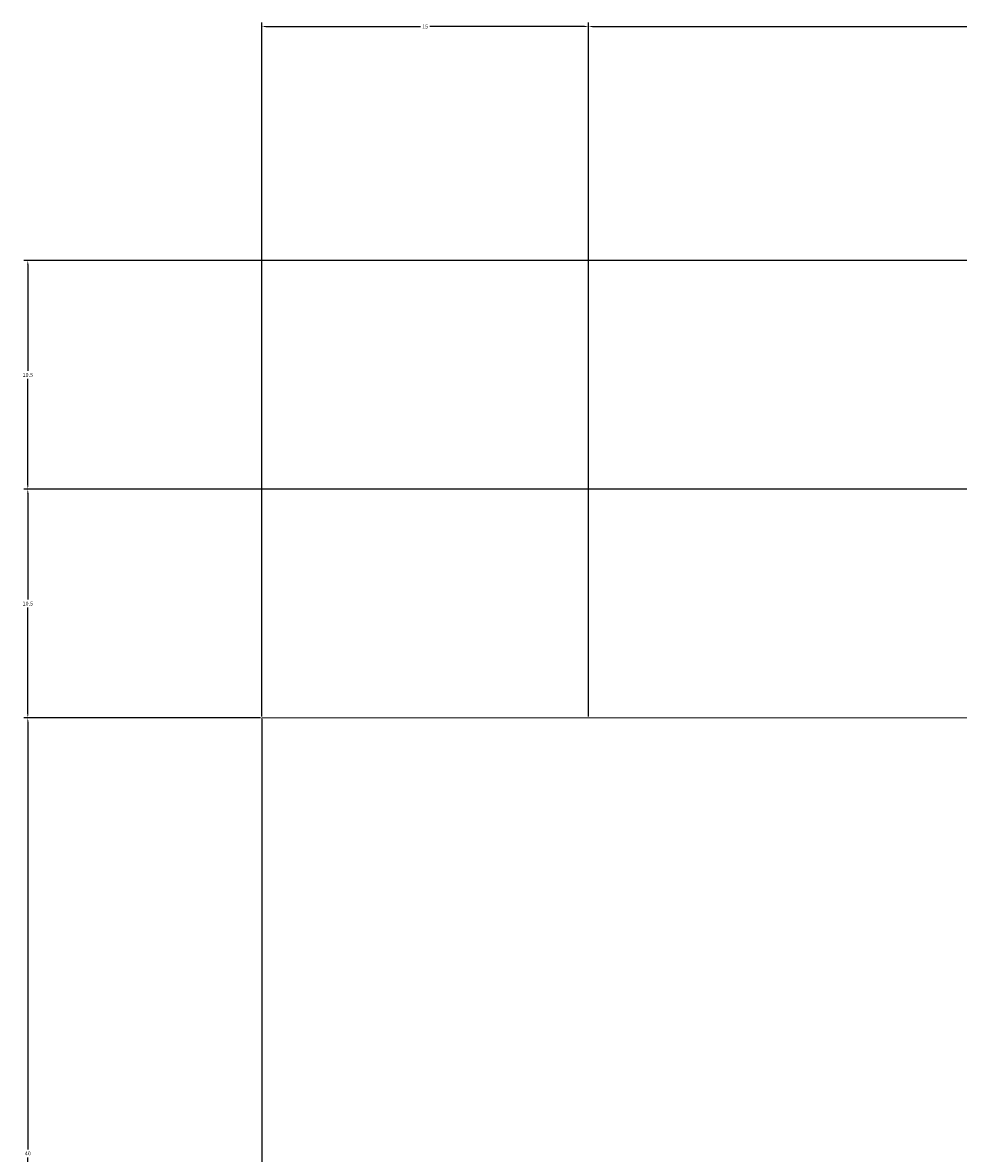
# Model space of a CAD drawing. Units: millimetres. Extents: x 315 to 487, y -72 to 32.
# Tile 2 of 4: x 315 to 358, y -20 to 32. Entities that reach past the tile are written whole.
import ezdxf

# ---------------------------------------------------------------- set-up
doc = ezdxf.new("R2010")
doc.units = ezdxf.units.MM
doc.layers.add('M-CONS', color=8, linetype='Continuous', lineweight=13)
doc.layers.add('M-DIMS', color=2, linetype='Continuous', lineweight=18)
doc.styles.get("Standard").update_dxf_attribs({"font": 'arial.ttf'})
doc.dimstyles.get("Standard").update_dxf_attribs({"dimtxt": 0.18, "dimasz": 0.18, "dimexe": 0.18, "dimexo": 0.0625, "dimgap": 0.09, "dimtad": 0, "dimtih": 1, "dimtoh": 1, "dimdec": 4, "dimzin": 0, "dimdsep": 46, "dimtxsty": 'Standard', "dimcen": 0.09, "dimadec": 0, "dimazin": 0, "dimtfac": 1, "dimtdec": 4, "dimtofl": 0, "dimtmove": 0, "dimatfit": 3, "dimfxl": 1, "dimtolj": 1, "dimtzin": 0, "dimarcsym": 0})

# ---------------------------------------------------------------- blocks, each defined once
blk = doc.blocks.new('*D3')
at = {"layer": 'Defpoints', "color": 0, "transparency": 16777216}
for p in [(326.007, 0), (476.007, 0), (476.007, -71.75)]:
    blk.add_point(p, dxfattribs=at)
at = {"layer": 'M-DIMS', "color": 0, "lineweight": -2, "transparency": 16777216}
for p, q in [((326.007, -0.062), (326.007, -71.93)), ((476.007, -0.062), (476.007, -71.93)), ((326.187, -71.75), (400.727, -71.75)), ((475.827, -71.75), (401.287, -71.75))]:
    blk.add_line(p, q, dxfattribs=at)
at = {"layer": 'M-DIMS', "color": 0, "transparency": 16777216}
for points in [[(326.187, -71.72), (326.187, -71.78), (326.007, -71.75)], [(475.827, -71.72), (475.827, -71.78), (476.007, -71.75)]]:
    blk.add_solid(points, dxfattribs=at)
at = {"layer": 'M-DIMS', "color": 0, "transparency": 16777216, "insert": (401.007, -71.75), "char_height": 0.18, "attachment_point": 5}
blk.add_mtext('\\A1;150', dxfattribs=at)
blk = doc.blocks.new('*D5')
at = {"layer": 'Defpoints', "color": 0, "transparency": 16777216}
for p in [(341.007, 31.75), (326.007, 0), (341.007, 0)]:
    blk.add_point(p, dxfattribs=at)
at = {"layer": 'M-DIMS', "color": 0, "lineweight": -2, "transparency": 16777216}
for p, q in [((326.007, 0.062), (326.007, 31.93)), ((326.187, 31.75), (333.296, 31.75)), ((340.827, 31.75), (333.719, 31.75)), ((341.007, 0.062), (341.007, 31.93))]:
    blk.add_line(p, q, dxfattribs=at)
at = {"layer": 'M-DIMS', "color": 0, "transparency": 16777216}
for points in [[(326.187, 31.78), (326.187, 31.72), (326.007, 31.75)], [(340.827, 31.78), (340.827, 31.72), (341.007, 31.75)]]:
    blk.add_solid(points, dxfattribs=at)
at = {"layer": 'M-DIMS', "color": 0, "transparency": 16777216, "insert": (333.507, 31.75), "char_height": 0.18, "attachment_point": 5}
blk.add_mtext('\\A1;15', dxfattribs=at)
blk = doc.blocks.new('*D6')
at = {"layer": 'Defpoints', "color": 0, "transparency": 16777216}
for p in [(386.007, 31.75), (386.007, 10.5), (341.007, 0)]:
    blk.add_point(p, dxfattribs=at)
at = {"layer": 'M-DIMS', "color": 0, "lineweight": -2, "transparency": 16777216}
for p, q in [((341.007, 0.062), (341.007, 31.93)), ((341.187, 31.75), (363.284, 31.75)), ((385.827, 31.75), (363.731, 31.75)), ((386.007, 10.562), (386.007, 31.93))]:
    blk.add_line(p, q, dxfattribs=at)
at = {"layer": 'M-DIMS', "color": 0, "transparency": 16777216}
for points in [[(341.187, 31.78), (341.187, 31.72), (341.007, 31.75)], [(385.827, 31.78), (385.827, 31.72), (386.007, 31.75)]]:
    blk.add_solid(points, dxfattribs=at)
at = {"layer": 'M-DIMS', "color": 0, "transparency": 16777216, "insert": (363.507, 31.75), "char_height": 0.18, "attachment_point": 5}
blk.add_mtext('\\A1;45', dxfattribs=at)
blk = doc.blocks.new('*D10')
at = {"layer": 'Defpoints', "color": 0, "transparency": 16777216}
for p in [(326.007, 0), (315.257, 0), (326.007, -40)]:
    blk.add_point(p, dxfattribs=at)
at = {"layer": 'M-DIMS', "color": 0, "lineweight": -2, "transparency": 16777216}
for p, q in [((325.945, 0), (315.077, 0)), ((315.257, -0.18), (315.257, -19.818)), ((315.257, -39.82), (315.257, -20.182)), ((325.945, -40), (315.077, -40))]:
    blk.add_line(p, q, dxfattribs=at)
at = {"layer": 'M-DIMS', "color": 0, "transparency": 16777216}
for points in [[(315.227, -0.18), (315.287, -0.18), (315.257, 0)], [(315.227, -39.82), (315.287, -39.82), (315.257, -40)]]:
    blk.add_solid(points, dxfattribs=at)
at = {"layer": 'M-DIMS', "color": 0, "transparency": 16777216, "insert": (315.257, -20), "char_height": 0.18, "attachment_point": 5}
blk.add_mtext('\\A1;40', dxfattribs=at)
blk = doc.blocks.new('*D11')
at = {"layer": 'Defpoints', "color": 0, "transparency": 16777216}
for p in [(315.257, 10.5), (386.007, 10.5), (326.007, 0)]:
    blk.add_point(p, dxfattribs=at)
at = {"layer": 'M-DIMS', "color": 0, "lineweight": -2, "transparency": 16777216}
for p, q in [((385.945, 10.5), (315.077, 10.5)), ((315.257, 10.32), (315.257, 5.432)), ((315.257, 0.18), (315.257, 5.068)), ((325.945, 0), (315.077, 0))]:
    blk.add_line(p, q, dxfattribs=at)
at = {"layer": 'M-DIMS', "color": 0, "transparency": 16777216}
for points in [[(315.227, 10.32), (315.287, 10.32), (315.257, 10.5)], [(315.227, 0.18), (315.287, 0.18), (315.257, 0)]]:
    blk.add_solid(points, dxfattribs=at)
at = {"layer": 'M-DIMS', "color": 0, "transparency": 16777216, "insert": (315.257, 5.25), "char_height": 0.18, "attachment_point": 5}
blk.add_mtext('\\A1;10.5', dxfattribs=at)
blk = doc.blocks.new('*D12')
at = {"layer": 'Defpoints', "color": 0, "transparency": 16777216}
for p in [(315.257, 21), (446.007, 21), (386.007, 10.5)]:
    blk.add_point(p, dxfattribs=at)
at = {"layer": 'M-DIMS', "color": 0, "lineweight": -2, "transparency": 16777216}
for p, q in [((445.945, 21), (315.077, 21)), ((315.257, 20.82), (315.257, 15.932)), ((315.257, 10.68), (315.257, 15.568)), ((385.945, 10.5), (315.077, 10.5))]:
    blk.add_line(p, q, dxfattribs=at)
at = {"layer": 'M-DIMS', "color": 0, "transparency": 16777216}
for points in [[(315.227, 20.82), (315.287, 20.82), (315.257, 21)], [(315.227, 10.68), (315.287, 10.68), (315.257, 10.5)]]:
    blk.add_solid(points, dxfattribs=at)
at = {"layer": 'M-DIMS', "color": 0, "transparency": 16777216, "insert": (315.257, 15.75), "char_height": 0.18, "attachment_point": 5}
blk.add_mtext('\\A1;10.5', dxfattribs=at)

msp = doc.modelspace()

# ---------------------------------------------------------------- linework, layer by layer
at = {"layer": 'M-CONS', "extrusion": (0, -1, 0)}
for p, q in [((326.007, 0, 190.054), (476.007, 0, 190.054)), ((466.007, 0, 200.054), (326.007, 0, 200.054)), ((326.007, 0, 200.054), (326.007, 0, 190.054)), ((326.007, 0, 200.054), (341.007, 0, 200.054)), ((326.007, 0, 200.054), (326.007, 0, 207.554)), ((434.007, 0, 240.054), (338.273, 0, 222.303))]:
    msp.add_line(p, q, dxfattribs=at)
at = {"layer": 'M-CONS', "extrusion": (0, 1, 0)}
msp.add_line((326.007, 0, 200.054), (326.007, -40, 200.054), dxfattribs=at)
at = {"layer": 'M-CONS', "extrusion": (0, -1, 0)}
msp.add_circle((341.007, 207.554), 3.5, dxfattribs=at)
msp.add_arc((341.007, 207.554), 15, 100.5046, 180, dxfattribs=at)

# ---------------------------------------------------------------- dimensions: what is measured, and where the dimension line sits
at = {"layer": 'M-DIMS'}
for base, p1, p2, picture, middle in [((341.007, 31.75), (326.007, 0), (341.007, 0), '*D5', (333.507, 31.75)), ((386.007, 31.75), (341.007, 0), (386.007, 10.5), '*D6', (363.507, 31.75)), ((476.007, -71.75), (326.007, 0), (476.007, 0), '*D3', (401.007, -71.75))]:
    dim = msp.add_linear_dim(base=base, p1=p1, p2=p2, dimstyle='Standard', override={"dimdec": 0, "dimlfac": 1, "dimrnd": 0, "dimzin": 0, "dimdsep": 46, "dimlunit": 2}, dxfattribs=at)
    dim.commit()
    dim.dimension.update_dxf_attribs({"geometry": picture, "text_midpoint": middle})
for base, p1, p2, override, picture, middle in [((315.257, 21), (386.007, 10.5), (446.007, 21), {"dimdec": 1, "dimlfac": 1, "dimrnd": 0, "dimzin": 0, "dimdsep": 46, "dimlunit": 2}, '*D12', (315.257, 15.75)), ((315.257, 10.5), (326.007, 0), (386.007, 10.5), {"dimdec": 1, "dimlfac": 1, "dimrnd": 0, "dimzin": 0, "dimdsep": 46, "dimlunit": 2}, '*D11', (315.257, 5.25)), ((315.257, 0), (326.007, -40), (326.007, 0), {"dimdec": 0, "dimlfac": 1, "dimrnd": 0, "dimzin": 0, "dimdsep": 46, "dimlunit": 2}, '*D10', (315.257, -20))]:
    dim = msp.add_linear_dim(base=base, p1=p1, p2=p2, angle=90, dimstyle='Standard', override=override, dxfattribs=at)
    dim.commit()
    dim.dimension.update_dxf_attribs({"geometry": picture, "text_midpoint": middle})

doc.saveas('drawing.dxf')
